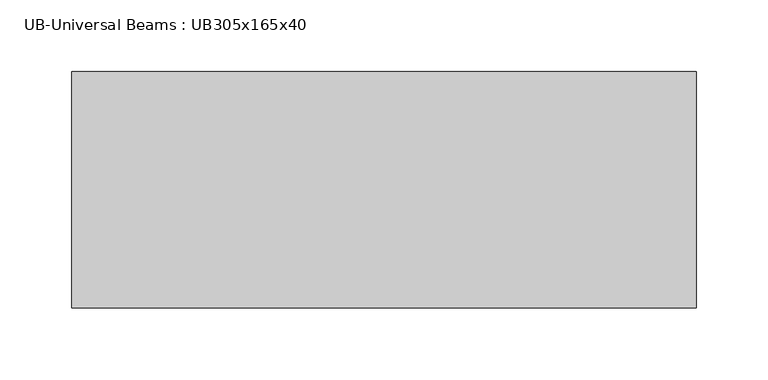
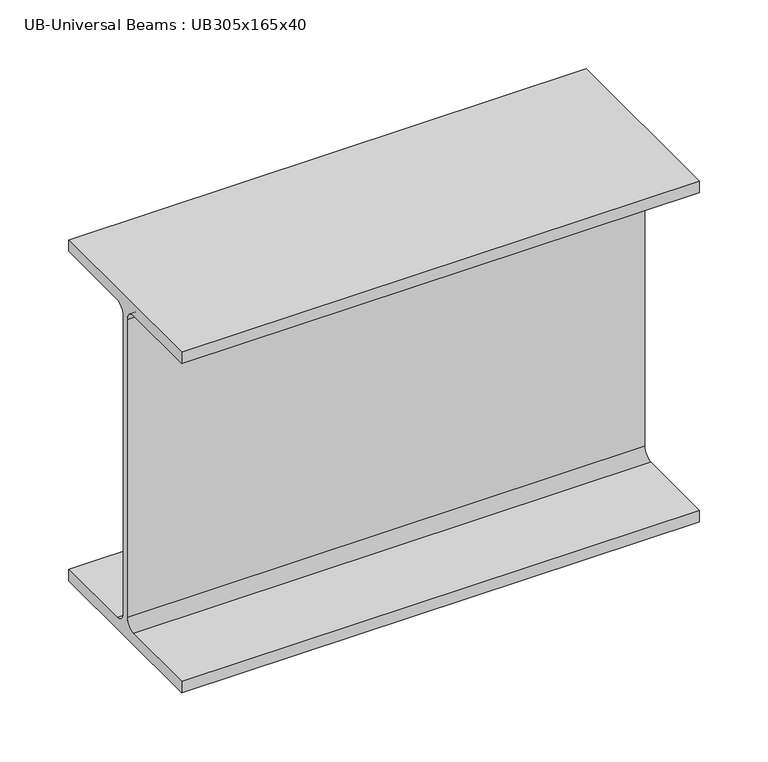
"""IFC4 building model written with IfcOpenShell, lengths in millimetres: beam geometry, UB-Universal Beams : UB305x165x40."""

from ifc_helpers import new_model, si_unit, point, frame, frame_2d, origin, place, context, project, spatial, polyline, circle_curve, trimmed, segment, composite_curve, outline, extrude, source, transform, mapped, element, save


def ub_universal_beams_ub305x165x40_63d5ebb1(model_context):
    return source(origin(), model_context, "Body", "SweptSolid", [
        extrude(outline(composite_curve([segment(polyline([(82.5, -141.5), (82.5, -151.7), (-82.5, -151.7), (-82.5, -141.5), (-11.9, -141.5)]), True, "CONTINUOUS"), segment(trimmed(circle_curve(frame_2d((-11.9, -132.6)), 8.9), [point((-11.9, -141.5))], [point((-3.0, -132.6))], True, "CARTESIAN"), True, "CONTINUOUS"), segment(polyline([(-3.0, -132.6), (-3.0, 132.6)]), True, "CONTINUOUS"), segment(trimmed(circle_curve(frame_2d((-11.9, 132.6)), 8.9), [point((-3.0, 132.6))], [point((-11.9, 141.5))], True, "CARTESIAN"), True, "CONTINUOUS"), segment(polyline([(-11.9, 141.5), (-82.5, 141.5), (-82.5, 151.7), (82.5, 151.7), (82.5, 141.5), (11.9, 141.5)]), True, "CONTINUOUS"), segment(trimmed(circle_curve(frame_2d((11.9, 132.6)), 8.9), [point((11.9, 141.5))], [point((3.0, 132.6))], True, "CARTESIAN"), True, "CONTINUOUS"), segment(polyline([(3.0, 132.6), (3.0, -132.6)]), True, "CONTINUOUS"), segment(trimmed(circle_curve(frame_2d((11.9, -132.6)), 8.9), [point((3.0, -132.6))], [point((11.9, -141.5))], True, "CARTESIAN"), True, "CONTINUOUS"), segment(polyline([(11.9, -141.5), (82.5, -141.5)]), True, "CONTINUOUS")], self_intersect=False)), frame((-204.9, 0.0, 0.0), z_axis=(1.0, 0.0, 0.0), x_axis=(0.0, 1.0, 0.0)), (0.0, 0.0, 1.0), 435.6),
    ])


if __name__ == "__main__":
    model = new_model("IFC4")
    model_context = context("Model", 3, world=origin())
    ifc_project = project(units=[si_unit("LENGTHUNIT", "METRE", prefix="MILLI")], contexts=[model_context])
    site = spatial("IfcSite", under=ifc_project)
    building = spatial("IfcBuilding", under=site)
    placement = place(None, origin())
    ub_universal_beams_ub305x165x40_shape = ub_universal_beams_ub305x165x40_63d5ebb1(model_context)
    element("IfcBeam", 1, ObjectType="UB-Universal Beams : UB305x165x40", at=placement, inside=building, context=model_context, shape_type="MappedRepresentation", body=[
        mapped(ub_universal_beams_ub305x165x40_shape, transform((0.0, 0.0, 0.0), x_axis=(1.0, 0.0, 0.0), y_axis=(0.0, 1.0, 0.0), z_axis=(0.0, 0.0, 1.0))),
    ])
    save(model, "model.ifc")

# Revit data of these elements
# Type "UB-Universal Beams : UB305x165x40"
#   Section Name Key = "UB305X165X40"
#   Width = 16.5 cm
#   Web Thickness = 0.6 cm
#   Web Fillet = 0.89 cm
#   Warping Constant = 164000.0 cm⁶
#   Torsional Moment of Inertia = 14.70 cm⁴
#   Section Area = 51.3 cm²
#   Plastic Modulus weak axis = 142.0 cm³
#   Plastic Modulus strong axis = 623.0 cm³
#   Nominal Weight = 40.2999 kgf/m
#   Moment of Inertia weak axis = 764.00 cm⁴
#   Moment of Inertia strong axis = 8503.00 cm⁴
#   Height = 30.34 cm
#   Flange Thickness = 1.02 cm
#   Elastic Modulus weak axis = 92.6 cm³
#   Elastic Modulus strong axis = 560.0 cm³
#   Centroid Vertical = 15.17 cm
#   Centroid Horizontal = 8.25 cm
#   Bolt Spacing = 9.0 cm
#   Length [instance default] = 1500 mm
#   Structural Material [instance default] = Metal - Steel 43-275
#   Type Comments = ""
#   Assembly Code = ""
# Element 1 (IfcBeam, "UB-Universal Beams : UB305x165x40")
#   Materials on its faces: "Metal - Steel 43-275"
# Materials
#   "Metal - Steel 43-275": class "Metal", colour RGB 247 247 247, transparency 0, Cost = 0
